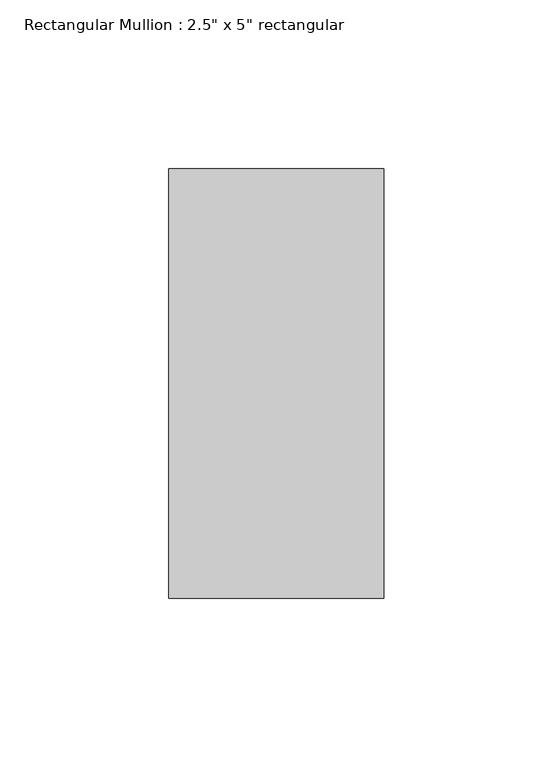
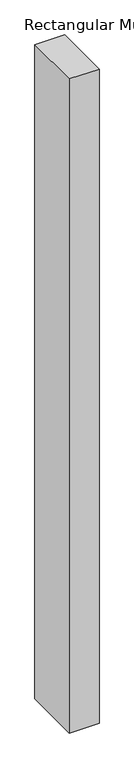
"""IFC4 building model written with IfcOpenShell, lengths in millimetres: member geometry."""

from ifc_helpers import new_model, si_unit, frame, origin, place, context, project, spatial, polyline, outline, extrude, source, transform, mapped, element, save


def member_7d2014ad(model_context):
    return source(origin(), model_context, "Body", "SweptSolid", [
        extrude(outline(polyline([(31.75, 63.5), (31.75, -63.5), (-31.75, -63.5), (-31.75, 63.5), (31.75, 63.5)])), frame((0.0, 0.0, -1475.7058851), z_axis=(0.0, 0.0, 1.0), x_axis=(1.0, 0.0, 0.0)), (0.0, 0.0, 1.0), 1475.7058851),
    ])


if __name__ == "__main__":
    model = new_model("IFC4")
    model_context = context("Model", 3, world=origin())
    ifc_project = project(units=[si_unit("LENGTHUNIT", "METRE", prefix="MILLI")], contexts=[model_context])
    site = spatial("IfcSite", under=ifc_project)
    building = spatial("IfcBuilding", under=site)
    placement = place(None, origin())
    member_shape = member_7d2014ad(model_context)
    element("IfcMember", 1, ObjectType="Rectangular Mullion : 2.5\" x 5\" rectangular", at=placement, inside=building, context=model_context, shape_type="MappedRepresentation", body=[
        mapped(member_shape, transform((0.0, 0.0, 0.0), x_axis=(1.0, 0.0, 0.0), y_axis=(0.0, 1.0, 0.0), z_axis=(0.0, 0.0, 1.0))),
    ])
    save(model, "model.ifc")

# Revit data of these elements
# Type "Rectangular Mullion : 2.5\" x 5\" rectangular"
#   built-in parameter 1007304 = 0.416667 (stored number, unit not read)
#   built-in parameter 1007301 = 0.104167 (stored number, unit not read)
#   built-in parameter 1007300 = 0.104167 (stored number, unit not read)
# Element 1 (IfcMember, "Rectangular Mullion : 2.5\" x 5\" rectangular")
#   Materials on its faces: "Aluminum"
# Materials
#   "Aluminum": class "Metal", colour RGB 247 247 247, transparency 0, Description = "Aluminum 6061", Cost = 0
